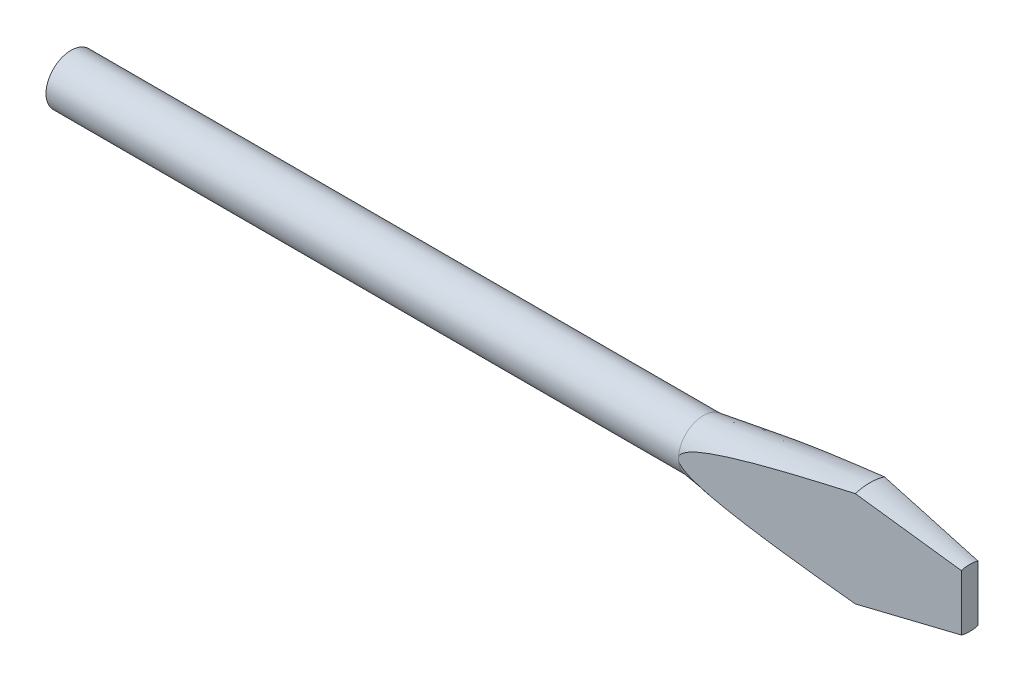
from build123d import *

# Parameters (mm, degrees)
BLADE_FLAT_CUT_DEPTH = 10


with BuildPart() as part:
    # Shaft Profile Sketch → Shaft Revolve (revolve)
    with BuildSketch(Plane.XY, mode=Mode.PRIVATE) as shaft_revolve_sk:
        Polygon((0, 0), (0, 3), (76, 3), (96, 6), (108, 3.5), (108, 0), align=None)
    revolve(shaft_revolve_sk.sketch.rotate(Axis((-206.404998063, 0, 0), (1, 0, 0)), 90), axis=Axis((-206.404998063, 0, 0), (1, 0, 0)))

    # Blade Flat Sketch → Blade Flat Cut (cut, symmetric)
    with BuildSketch(Plane(origin=(0, 0, 0), x_dir=(1, 0, 0), z_dir=(0, 1, 0))):
        Polygon((108, 1), (76, 3), (76, 10.728035522), (108, 10.728035522), align=None)
    blade_flat_cut = extrude(amount=BLADE_FLAT_CUT_DEPTH, both=True, mode=Mode.SUBTRACT)

    # Blade Flat Mirror: Blade Flat Cut across plane
    add(blade_flat_cut.mirror(Plane.XY), mode=Mode.SUBTRACT)


solid = part.part
